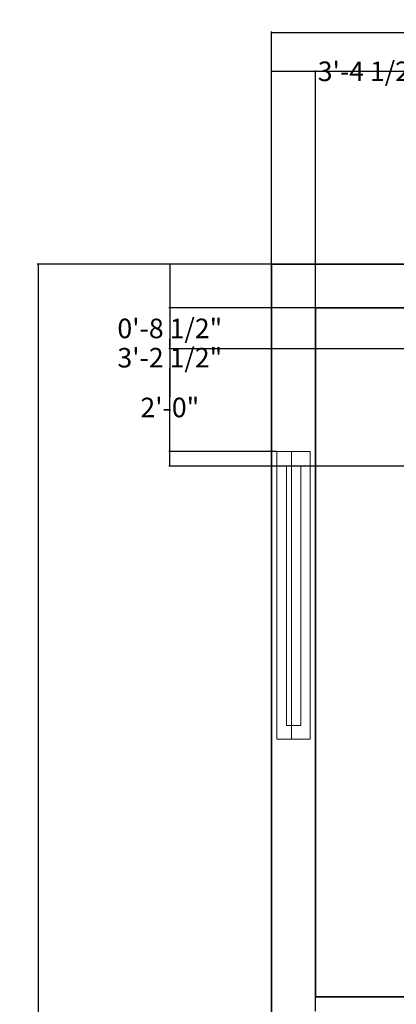
# Model space of a CAD drawing. Units: inches. Extents: x 311 to 754, y 60 to 497.
# Tile 2 of 11: x 311 to 388, y 296 to 497. Entities that reach past the tile are written whole.
import ezdxf

# ---------------------------------------------------------------- set-up
doc = ezdxf.new("R2010")
doc.units = ezdxf.units.IN
doc.header["$MEASUREMENT"] = 0
for name, color, linetype, lineweight in [('A-ANNO-DIMS', 2, 'Continuous', 18), ('A-WALL', 7, 'Continuous', 35), ('windows', 120, 'Continuous', 18)]:
    doc.layers.add(name, color=color, linetype=linetype, lineweight=lineweight)
doc.styles.get("Standard").update_dxf_attribs({"font": 'arial.ttf'})
doc.dimstyles.get("Standard").update_dxf_attribs({"dimtxt": 4, "dimasz": 0.18, "dimexe": 0.18, "dimexo": 0.0625, "dimgap": 0.09, "dimtad": 0, "dimtih": 1, "dimtoh": 1, "dimdec": 0, "dimrnd": 6, "dimzin": 0, "dimdsep": 46, "dimlunit": 3, "dimtxsty": 'Standard', "dimcen": 0.09, "dimadec": 0, "dimazin": 0, "dimtfac": 1, "dimtdec": 0, "dimtofl": 0, "dimtmove": 0, "dimatfit": 3, "dimfxl": 1, "dimtolj": 1, "dimtzin": 0, "dimarcsym": 0})

# ---------------------------------------------------------------- blocks, each defined once
blk = doc.blocks.new('*D103')
at = {"layer": 'A-ANNO-DIMS', "color": 0, "lineweight": -2, "transparency": 16777216}
for p, q in [((362.8, 447.3), (362.8, 494.8)), ((362.98, 494.62), (539.32, 494.62)), ((722.62, 494.62), (546.29, 494.62)), ((722.8, 447.3), (722.8, 494.8))]:
    blk.add_line(p, q, dxfattribs=at)
at = {"layer": 'A-ANNO-DIMS', "color": 0, "transparency": 16777216}
for points in [[(362.98, 494.65), (362.98, 494.59), (362.8, 494.62)], [(722.62, 494.65), (722.62, 494.59), (722.8, 494.62)]]:
    blk.add_solid(points, dxfattribs=at)
at = {"layer": 'Defpoints', "color": 0, "transparency": 16777216}
for p in [(722.8, 494.62), (362.8, 447.24), (722.8, 447.24)]:
    blk.add_point(p, dxfattribs=at)
at = {"layer": 'A-ANNO-DIMS', "color": 0, "transparency": 16777216, "insert": (542.8, 494.62), "char_height": 4, "attachment_point": 5}
blk.add_mtext("\\A1;30'", dxfattribs=at)
blk = doc.blocks.new('*D104')
at = {"layer": 'A-ANNO-DIMS', "color": 0, "lineweight": -2, "transparency": 16777216}
for p, q in [((362.74, 447.24), (314.86, 447.24)), ((315.04, 447.06), (315.04, 269.37)), ((315.04, 87.42), (315.04, 265.1)), ((362.74, 87.24), (314.86, 87.24))]:
    blk.add_line(p, q, dxfattribs=at)
at = {"layer": 'A-ANNO-DIMS', "color": 0, "transparency": 16777216}
for points in [[(315.01, 447.06), (315.07, 447.06), (315.04, 447.24)], [(315.01, 87.42), (315.07, 87.42), (315.04, 87.24)]]:
    blk.add_solid(points, dxfattribs=at)
at = {"layer": 'Defpoints', "color": 0, "transparency": 16777216}
for p in [(362.8, 447.24), (315.04, 87.24), (362.8, 87.24)]:
    blk.add_point(p, dxfattribs=at)
at = {"layer": 'A-ANNO-DIMS', "color": 0, "transparency": 16777216, "insert": (315.04, 267.24), "char_height": 4, "attachment_point": 5}
blk.add_mtext("\\A1;30'", dxfattribs=at)
blk = doc.blocks.new('WIN-FRAME-59IN')
for points in [[(0, 0), (0, 6.8), (58.92, 6.8), (58.92, 0)], [(2.85, 4.84), (55.97, 4.84), (55.97, 1.89), (2.85, 1.89)]]:
    blk.add_lwpolyline(points, close=True)
blk = doc.blocks.new('*D118')
at = {"layer": 'A-ANNO-DIMS', "color": 0, "lineweight": -2, "transparency": 16777216}
for p, q in [((362.8, 447.3), (362.8, 486.86)), ((362.98, 486.68), (372.96, 486.68)), ((403.08, 486.68), (393.1, 486.68)), ((403.26, 439.39), (403.26, 486.86))]:
    blk.add_line(p, q, dxfattribs=at)
at = {"layer": 'A-ANNO-DIMS', "color": 0, "transparency": 16777216}
for points in [[(362.98, 486.71), (362.98, 486.65), (362.8, 486.68)], [(403.08, 486.71), (403.08, 486.65), (403.26, 486.68)]]:
    blk.add_solid(points, dxfattribs=at)
at = {"layer": 'Defpoints', "color": 0, "transparency": 16777216}
for p in [(403.26, 486.68), (362.8, 447.24), (403.26, 439.33)]:
    blk.add_point(p, dxfattribs=at)
at = {"layer": 'A-ANNO-DIMS', "color": 0, "transparency": 16777216, "insert": (383.03, 486.68), "char_height": 4, "attachment_point": 5}
blk.add_mtext('\\A1;3\'-4 1/2"', dxfattribs=at)
blk = doc.blocks.new('*D124')
at = {"layer": 'A-ANNO-DIMS', "color": 0, "lineweight": -2, "transparency": 16777216}
for p, q in [((362.74, 447.24), (341.82, 447.24)), ((342, 447.06), (342, 430.23)), ((342, 409.07), (342, 425.91)), ((363.84, 408.89), (341.82, 408.89))]:
    blk.add_line(p, q, dxfattribs=at)
at = {"layer": 'A-ANNO-DIMS', "color": 0, "transparency": 16777216}
for points in [[(341.97, 447.06), (342.03, 447.06), (342, 447.24)], [(341.97, 409.07), (342.03, 409.07), (342, 408.89)]]:
    blk.add_solid(points, dxfattribs=at)
at = {"layer": 'Defpoints', "color": 0, "transparency": 16777216}
for p in [(362.8, 447.24), (342, 408.89), (363.9, 408.89)]:
    blk.add_point(p, dxfattribs=at)
at = {"layer": 'A-ANNO-DIMS', "color": 0, "transparency": 16777216, "insert": (342, 428.07), "char_height": 4, "attachment_point": 5}
blk.add_mtext('\\A1;3\'-2 1/2"', dxfattribs=at)
blk = doc.blocks.new('*D136')
at = {"layer": 'A-ANNO-DIMS', "color": 0, "lineweight": -2, "transparency": 16777216}
for p, q in [((371.8, 294.3), (371.8, 486.86)), ((371.98, 486.68), (405.39, 486.68)), ((449.62, 486.68), (416.22, 486.68)), ((449.8, 294.3), (449.8, 486.86))]:
    blk.add_line(p, q, dxfattribs=at)
at = {"layer": 'A-ANNO-DIMS', "color": 0, "transparency": 16777216}
for points in [[(371.98, 486.71), (371.98, 486.65), (371.8, 486.68)], [(449.62, 486.71), (449.62, 486.65), (449.8, 486.68)]]:
    blk.add_solid(points, dxfattribs=at)
at = {"layer": 'Defpoints', "color": 0, "transparency": 16777216}
for p in [(371.8, 486.68), (371.8, 294.24), (449.8, 294.24)]:
    blk.add_point(p, dxfattribs=at)
at = {"layer": 'A-ANNO-DIMS', "color": 0, "transparency": 16777216, "insert": (410.8, 486.68), "char_height": 4, "attachment_point": 5}
blk.add_mtext('\\A1;6\'-6"', dxfattribs=at)
blk = doc.blocks.new('*D145')
at = {"layer": 'A-ANNO-DIMS', "color": 0, "lineweight": -2, "transparency": 16777216}
for p, q in [((500.37, 429.88), (341.82, 429.88)), ((342, 429.7), (342, 420.01)), ((342, 406.06), (342, 415.74)), ((504.87, 405.88), (341.82, 405.88))]:
    blk.add_line(p, q, dxfattribs=at)
at = {"layer": 'A-ANNO-DIMS', "color": 0, "transparency": 16777216}
for points in [[(341.97, 429.7), (342.03, 429.7), (342, 429.88)], [(341.97, 406.06), (342.03, 406.06), (342, 405.88)]]:
    blk.add_solid(points, dxfattribs=at)
at = {"layer": 'Defpoints', "color": 0, "transparency": 16777216}
for p in [(342, 429.88), (500.44, 429.88), (504.94, 405.88)]:
    blk.add_point(p, dxfattribs=at)
at = {"layer": 'A-ANNO-DIMS', "color": 0, "transparency": 16777216, "insert": (342, 417.88), "char_height": 4, "attachment_point": 5}
blk.add_mtext('\\A1;2\'-0"', dxfattribs=at)
blk = doc.blocks.new('*D151')
at = {"layer": 'A-ANNO-DIMS', "color": 0, "lineweight": -2, "transparency": 16777216}
for p, q in [((494.74, 438.24), (341.82, 438.24)), ((342, 438.06), (342, 436.22)), ((342, 430.06), (342, 431.9)), ((500.37, 429.88), (341.82, 429.88))]:
    blk.add_line(p, q, dxfattribs=at)
at = {"layer": 'A-ANNO-DIMS', "color": 0, "transparency": 16777216}
for points in [[(341.97, 438.06), (342.03, 438.06), (342, 438.24)], [(341.97, 430.06), (342.03, 430.06), (342, 429.88)]]:
    blk.add_solid(points, dxfattribs=at)
at = {"layer": 'Defpoints', "color": 0, "transparency": 16777216}
for p in [(494.8, 438.24), (342, 429.88), (500.44, 429.88)]:
    blk.add_point(p, dxfattribs=at)
at = {"layer": 'A-ANNO-DIMS', "color": 0, "transparency": 16777216, "insert": (342, 434.06), "char_height": 4, "attachment_point": 5}
blk.add_mtext('\\A1;0\'-8 1/2"', dxfattribs=at)

msp = doc.modelspace()

# ---------------------------------------------------------------- linework, layer by layer
at = {"layer": 'A-WALL'}
for p, q in [((722.8, 447.24), (362.8, 447.24)), ((362.8, 447.24), (362.8, 87.24)), ((371.8, 438.24), (371.8, 297.24)), ((491.8, 438.24), (371.8, 438.24)), ((494.8, 297.24), (371.8, 297.24))]:
    msp.add_line(p, q, dxfattribs=at)
at = {"layer": 'windows'}
for p, q in [((363.9, 408.89), (366.93, 408.89)), ((366.93, 408.89), (366.93, 349.98))]:
    msp.add_line(p, q, dxfattribs=at)

# ---------------------------------------------------------------- block references
at = {"layer": 'windows', "rotation": 90.00000000000011}
msp.add_blockref('WIN-FRAME-59IN', (370.71, 349.98), dxfattribs=at)

# ---------------------------------------------------------------- dimensions: what is measured, and where the dimension line sits
at = {"layer": 'A-ANNO-DIMS'}
for base, p1, p2, override, picture, middle in [((722.8, 494.62), (362.8, 447.24), (722.8, 447.24), {"dimclrd": 0, "dimclre": 0, "dimclrt": 0}, '*D103', (542.8, 494.62)), ((403.26, 486.68), (362.8, 447.24), (403.26, 439.33), {"dimdec": 1, "dimlfac": 1, "dimrnd": 0, "dimzin": 1, "dimdsep": 46, "dimlunit": 4, "dimfrac": 2}, '*D118', (383.03, 486.68)), ((371.8, 486.68), (449.8, 294.24), (371.8, 294.24), {"dimdec": 1, "dimlfac": 1, "dimrnd": 0, "dimzin": 1, "dimdsep": 46, "dimlunit": 4, "dimfrac": 2}, '*D136', (410.8, 486.68))]:
    dim = msp.add_linear_dim(base=base, p1=p1, p2=p2, dimstyle='Standard', override=override, dxfattribs=at)
    dim.commit()
    dim.dimension.update_dxf_attribs({"geometry": picture, "text_midpoint": middle})
for base, p1, p2, override, picture, middle in [((315.04, 87.24), (362.8, 447.24), (362.8, 87.24), {"dimclrd": 0, "dimclre": 0, "dimclrt": 0}, '*D104', (315.04, 267.24)), ((342.0046, 408.894), (362.8046, 447.2377), (363.9033, 408.894), {"dimdec": 1, "dimlfac": 1, "dimrnd": 0, "dimzin": 1, "dimdsep": 46, "dimlunit": 4, "dimfrac": 2}, '*D124', (342.0046, 428.0658)), ((342, 429.88), (494.8, 438.24), (500.44, 429.88), {"dimdec": 1, "dimlfac": 1, "dimrnd": 0, "dimzin": 1, "dimdsep": 46, "dimlunit": 4, "dimfrac": 2}, '*D151', (342, 434.06)), ((342, 429.88), (504.94, 405.88), (500.44, 429.88), {"dimdec": 1, "dimlfac": 1, "dimrnd": 0, "dimzin": 1, "dimdsep": 46, "dimlunit": 4, "dimfrac": 2}, '*D145', (342, 417.88))]:
    dim = msp.add_linear_dim(base=base, p1=p1, p2=p2, angle=90, dimstyle='Standard', override=override, dxfattribs=at)
    dim.commit()
    dim.dimension.update_dxf_attribs({"geometry": picture, "text_midpoint": middle})

doc.saveas('drawing.dxf')
